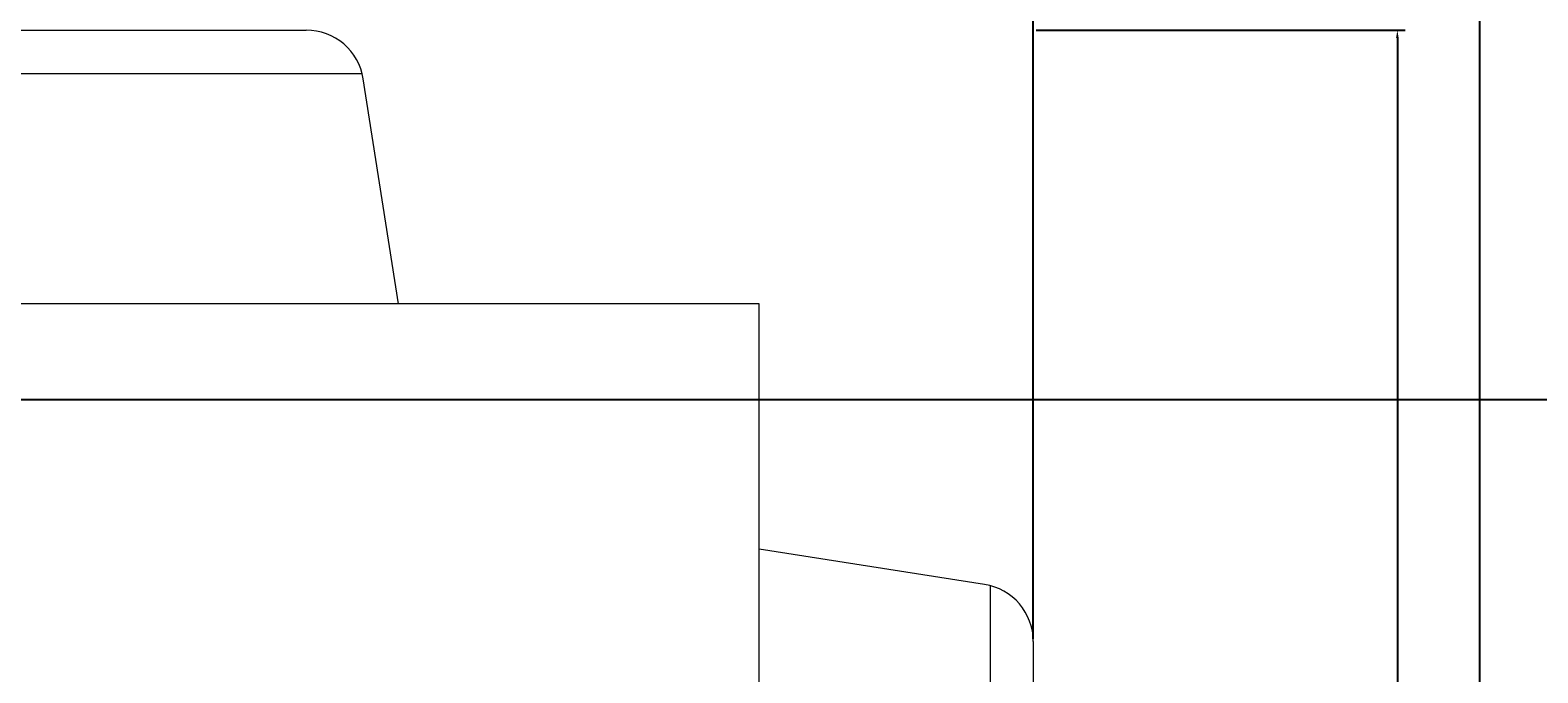
# Model space of a CAD drawing. Units: inches. Extents: x 2231 to 2461, y 2045 to 2455.
# Tile 28 of 95: x 2361 to 2396, y 2144 to 2159. Entities that reach past the tile are written whole.
import ezdxf

# ---------------------------------------------------------------- set-up
doc = ezdxf.new("R2010")
doc.units = ezdxf.units.IN
doc.layers.add('A-ANNO-DIMS', color=2, linetype='Continuous', lineweight=18)
doc.layers.add('A-FURN', color=9, linetype='Continuous', lineweight=18)
doc.styles.get("Standard").update_dxf_attribs({"font": 'arial.ttf'})
doc.dimstyles.get("Standard").update_dxf_attribs({"dimtxt": 0.18, "dimasz": 0.18, "dimexe": 0.18, "dimexo": 0.0625, "dimgap": 0.09, "dimtad": 0, "dimtih": 1, "dimtoh": 1, "dimdec": 4, "dimzin": 0, "dimdsep": 46, "dimtxsty": 'Standard', "dimcen": 0.09, "dimadec": 0, "dimazin": 0, "dimtfac": 1, "dimtdec": 4, "dimtofl": 0, "dimtmove": 0, "dimatfit": 3, "dimfxl": 1, "dimtolj": 1, "dimtzin": 0, "dimarcsym": 0})

# ---------------------------------------------------------------- blocks, each defined once
blk = doc.blocks.new('Dining Set - 36 x 72 in.')
for p, q in [((0.874, 27.5), (13.451, 27.5)), ((-1.068, 26), (15.402, 26)), ((16.647, 17.998), (15.427, 25.809)), ((29.162, 18), (-4.062, 18)), ((29.162, -18), (29.162, 18)), ((36.971, 8.264), (29.16, 9.485)), ((37.162, 8.23), (37.162, -8.239)), ((38.662, 6.288), (38.662, -6.288))]:
    blk.add_line(p, q)
for centre, start, end in [((13.451, 25.5), 8.881, 90), ((36.662, 6.288), 0, 81.1194)]:
    blk.add_arc(centre, 2, start, end)
blk = doc.blocks.new('*D32')
at = {"layer": 'A-ANNO-DIMS', "color": 0, "lineweight": -2, "transparency": 16777216}
for p, q in [((2384.605, 2159.115), (2393.089, 2159.115)), ((2392.909, 2158.935), (2392.909, 2141.072)), ((2392.909, 2122.845), (2392.909, 2140.708)), ((2384.605, 2122.665), (2393.089, 2122.665))]:
    blk.add_line(p, q, dxfattribs=at)
at = {"layer": 'A-ANNO-DIMS', "color": 0, "transparency": 16777216}
for points in [[(2392.879, 2158.935), (2392.939, 2158.935), (2392.909, 2159.115)], [(2392.879, 2122.845), (2392.939, 2122.845), (2392.909, 2122.665)]]:
    blk.add_solid(points, dxfattribs=at)
at = {"layer": 'Defpoints', "color": 0, "transparency": 16777216}
for p in [(2384.543, 2159.115), (2392.909, 2159.115), (2384.543, 2122.665)]:
    blk.add_point(p, dxfattribs=at)
at = {"layer": 'A-ANNO-DIMS', "color": 0, "transparency": 16777216, "insert": (2392.909, 2140.89), "char_height": 0.18, "attachment_point": 5}
blk.add_mtext('\\A1;36', dxfattribs=at)
blk = doc.blocks.new('*D60')
at = {"layer": 'A-ANNO-DIMS', "color": 0, "lineweight": -2, "transparency": 16777216}
for p, q in [((2432.731, 2182.833), (2230.981, 2182.833)), ((2231.161, 2182.653), (2231.161, 2166.906)), ((2231.161, 2150.795), (2231.161, 2166.542)), ((2432.731, 2150.615), (2230.981, 2150.615))]:
    blk.add_line(p, q, dxfattribs=at)
at = {"layer": 'A-ANNO-DIMS', "color": 0, "transparency": 16777216}
for points in [[(2231.131, 2182.653), (2231.191, 2182.653), (2231.161, 2182.833)], [(2231.131, 2150.795), (2231.191, 2150.795), (2231.161, 2150.615)]]:
    blk.add_solid(points, dxfattribs=at)
at = {"layer": 'Defpoints', "color": 0, "transparency": 16777216}
for p in [(2231.161, 2182.833), (2432.794, 2182.833), (2432.794, 2150.615)]:
    blk.add_point(p, dxfattribs=at)
at = {"layer": 'A-ANNO-DIMS', "color": 0, "transparency": 16777216, "insert": (2231.161, 2166.724), "char_height": 0.18, "attachment_point": 5}
blk.add_mtext('\\A1;32.22', dxfattribs=at)
blk = doc.blocks.new('*D66')
at = {"layer": 'A-ANNO-DIMS', "color": 0, "lineweight": -2, "transparency": 16777216}
for p, q in [((2348.189, 2096.895), (2348.189, 2454.645)), ((2348.369, 2454.465), (2378.167, 2454.465)), ((2408.614, 2454.465), (2378.815, 2454.465)), ((2408.794, 2096.895), (2408.794, 2454.645))]:
    blk.add_line(p, q, dxfattribs=at)
at = {"layer": 'A-ANNO-DIMS', "color": 0, "transparency": 16777216}
for points in [[(2348.369, 2454.495), (2348.369, 2454.435), (2348.189, 2454.465)], [(2408.614, 2454.495), (2408.614, 2454.435), (2408.794, 2454.465)]]:
    blk.add_solid(points, dxfattribs=at)
at = {"layer": 'Defpoints', "color": 0, "transparency": 16777216}
for p in [(2408.794, 2454.465), (2348.189, 2096.833), (2408.794, 2096.833)]:
    blk.add_point(p, dxfattribs=at)
at = {"layer": 'A-ANNO-DIMS', "color": 0, "transparency": 16777216, "insert": (2378.491, 2454.465), "char_height": 0.18, "attachment_point": 5}
blk.add_mtext('\\A1;60.6', dxfattribs=at)
blk = doc.blocks.new('*D69')
at = {"layer": 'A-ANNO-DIMS', "color": 0, "lineweight": -2, "transparency": 16777216}
for p, q in [((2340.667, 2189.285), (2340.667, 2044.803)), ((2394.794, 2186.77), (2394.794, 2044.803)), ((2340.847, 2044.983), (2367.337, 2044.983)), ((2394.614, 2044.983), (2368.124, 2044.983))]:
    blk.add_line(p, q, dxfattribs=at)
at = {"layer": 'A-ANNO-DIMS', "color": 0, "transparency": 16777216}
for points in [[(2340.847, 2045.013), (2340.847, 2044.953), (2340.667, 2044.983)], [(2394.614, 2045.013), (2394.614, 2044.953), (2394.794, 2044.983)]]:
    blk.add_solid(points, dxfattribs=at)
at = {"layer": 'Defpoints', "color": 0, "transparency": 16777216}
for p in [(2340.667, 2189.348), (2394.794, 2186.833), (2394.794, 2044.983)]:
    blk.add_point(p, dxfattribs=at)
at = {"layer": 'A-ANNO-DIMS', "color": 0, "transparency": 16777216, "insert": (2367.73, 2044.983), "char_height": 0.18, "attachment_point": 5}
blk.add_mtext('\\A1;54.13', dxfattribs=at)
blk = doc.blocks.new('*D72')
at = {"layer": 'A-ANNO-DIMS', "color": 0, "lineweight": -2, "transparency": 16777216}
for p, q in [((2384.543, 2145.12), (2384.543, 2454.645)), ((2384.723, 2454.465), (2396.272, 2454.465)), ((2408.614, 2454.465), (2397.064, 2454.465)), ((2408.794, 2150.677), (2408.794, 2454.645))]:
    blk.add_line(p, q, dxfattribs=at)
at = {"layer": 'A-ANNO-DIMS', "color": 0, "transparency": 16777216}
for points in [[(2384.723, 2454.495), (2384.723, 2454.435), (2384.543, 2454.465)], [(2408.614, 2454.495), (2408.614, 2454.435), (2408.794, 2454.465)]]:
    blk.add_solid(points, dxfattribs=at)
at = {"layer": 'Defpoints', "color": 0, "transparency": 16777216}
for p in [(2408.794, 2454.465), (2408.794, 2150.615), (2384.543, 2145.058)]:
    blk.add_point(p, dxfattribs=at)
at = {"layer": 'A-ANNO-DIMS', "color": 0, "transparency": 16777216, "insert": (2396.668, 2454.465), "char_height": 0.18, "attachment_point": 5}
blk.add_mtext('\\A1;24.25', dxfattribs=at)

msp = doc.modelspace()

# ---------------------------------------------------------------- block references
at = {"layer": 'A-FURN', "xscale": 0.6627357546055535, "yscale": 0.6627357546055535, "zscale": 0.6627357546055535}
msp.add_blockref('Dining Set - 36 x 72 in.', (2358.9199, 2140.8902), dxfattribs=at)

# ---------------------------------------------------------------- dimensions: what is measured, and where the dimension line sits
at = {"layer": 'A-ANNO-DIMS'}
for base, p1, p2, override, picture, middle in [((2408.7935, 2454.4653), (2348.1888, 2096.8328), (2408.7935, 2096.8328), {"dimdec": 1, "dimlfac": 1, "dimrnd": 0, "dimzin": 0, "dimdsep": 46, "dimlunit": 2}, '*D66', (2378.4912, 2454.4653)), ((2408.7935, 2454.4653), (2384.5428, 2145.0576), (2408.7935, 2150.6145), {"dimdec": 2, "dimlfac": 1, "dimrnd": 0, "dimzin": 0, "dimdsep": 46, "dimlunit": 2}, '*D72', (2396.6682, 2454.4653)), ((2394.7935, 2044.9825), (2340.6673, 2189.3477), (2394.7935, 2186.8328), {"dimdec": 2, "dimlfac": 1, "dimrnd": 0, "dimzin": 0, "dimdsep": 46, "dimlunit": 2}, '*D69', (2367.7304, 2044.9825))]:
    dim = msp.add_linear_dim(base=base, p1=p1, p2=p2, dimstyle='Standard', override=override, dxfattribs=at)
    dim.commit()
    dim.dimension.update_dxf_attribs({"geometry": picture, "text_midpoint": middle})
for base, p1, p2, override, picture, middle in [((2231.161, 2182.8328), (2432.7935, 2150.6145), (2432.7935, 2182.8328), {"dimdec": 2, "dimlfac": 1, "dimrnd": 0, "dimzin": 0, "dimdsep": 46, "dimlunit": 2}, '*D60', (2231.161, 2166.7237)), ((2392.9094, 2159.1154), (2384.5428, 2122.665), (2384.5428, 2159.1154), {"dimdec": 0, "dimlfac": 1, "dimrnd": 0, "dimzin": 0, "dimdsep": 46, "dimlunit": 2}, '*D32', (2392.9094, 2140.8902))]:
    dim = msp.add_linear_dim(base=base, p1=p1, p2=p2, angle=90, dimstyle='Standard', override=override, dxfattribs=at)
    dim.commit()
    dim.dimension.update_dxf_attribs({"geometry": picture, "text_midpoint": middle})

doc.saveas('drawing.dxf')
